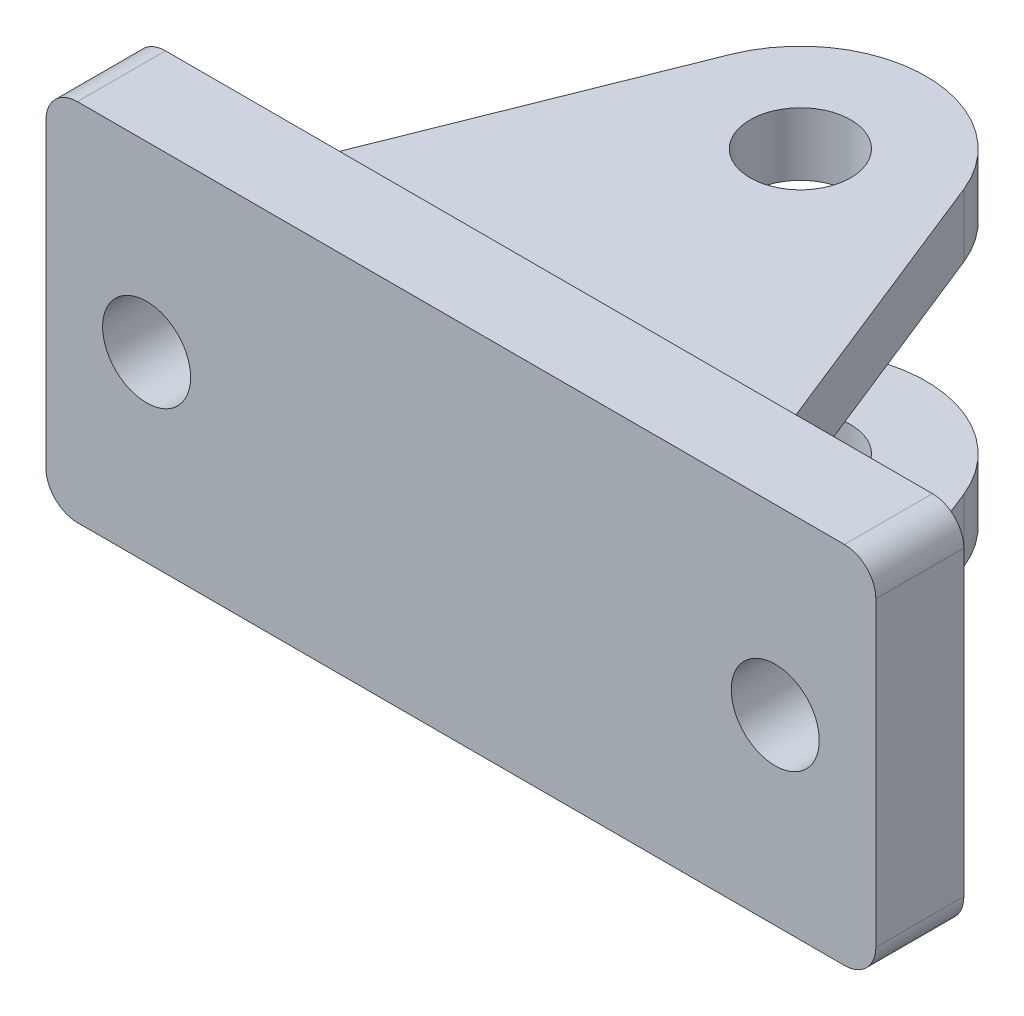
from build123d import *

# Parameters (mm, degrees)
BASE_PLATE_SKETCH_R = 7
BASE_PLATE_DEPTH    = 14
PIVOT_LUG_SKETCH_R  = 8
PIVOT_LUG_DEPTH     = 10


with BuildPart() as part:
    # Base Plate Sketch → Base Plate (new body)
    with BuildSketch(Plane.XY):
        with BuildLine():
            Line((-61, 29), (61, 29))
            ThreePointArc((61, 29), (64.535533906, 27.535533906), (66, 24))
            Line((66, 24), (66, -24))
            ThreePointArc((66, -24), (64.535533906, -27.535533906), (61, -29))
            Line((61, -29), (-61, -29))
            ThreePointArc((-61, -29), (-64.535533906, -27.535533906), (-66, -24))
            Line((-66, -24), (-66, 24))
            ThreePointArc((-66, 24), (-64.535533906, 27.535533906), (-61, 29))
        make_face()
        with Locations((-50, 0)):
            Circle(BASE_PLATE_SKETCH_R, mode=Mode.SUBTRACT)
        with Locations(Location((50, 0, 0), (0, 0, 180))):
            Circle(BASE_PLATE_SKETCH_R, mode=Mode.SUBTRACT)
    extrude(amount=BASE_PLATE_DEPTH)

    # Pivot Lug Sketch → Pivot Lug (add)
    with BuildSketch(Plane(origin=(0, 16, 0), x_dir=(1, 0, 0), z_dir=(0, 1, 0))):
        with BuildLine():
            Line((-37.5, 0), (37.5, 0))
            Line((37.5, 0), (18.575020612, 47.414081823))
            ThreePointArc((18.575020612, 47.414081823), (0, 60), (-18.575020612, 47.414081823))
            Line((-18.575020612, 47.414081823), (-37.5, 0))
        make_face()
        with Locations(Location((0, 40, 0), (0, 0, 270))):
            Circle(PIVOT_LUG_SKETCH_R, mode=Mode.SUBTRACT)
    pivot_lug = extrude(amount=PIVOT_LUG_DEPTH)

    # Pivot Lug Mirror: Pivot Lug across plane
    add(pivot_lug.mirror(Plane.ZX))


solid = part.part
